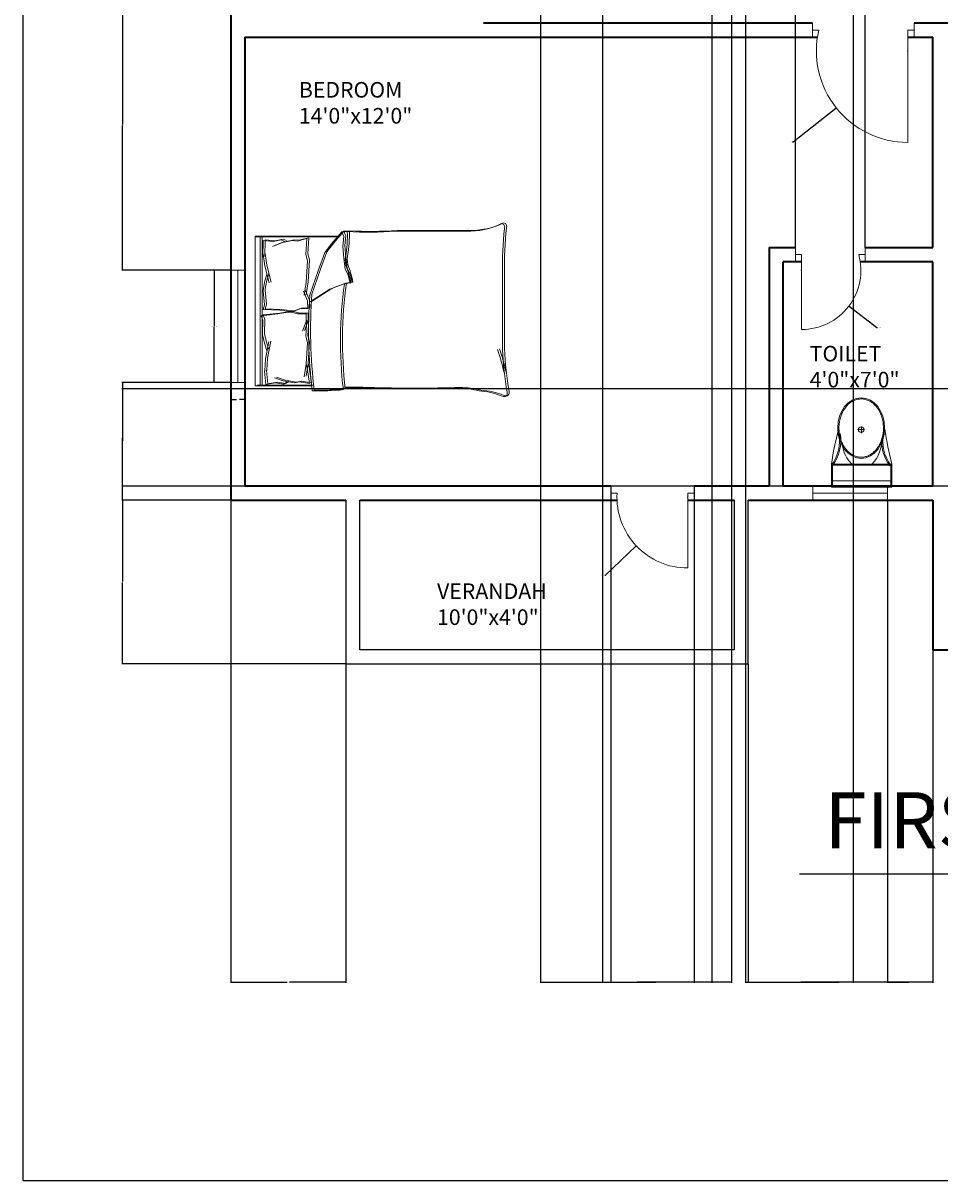
# Model space of a CAD drawing. Units: inches. Extents: x 1861 to 2564, y 1482 to 2317.
# Tile 1 of 11: x 1861 to 2155, y 1482 to 1853. Entities that reach past the tile are written whole.
import ezdxf

# ---------------------------------------------------------------- set-up
doc = ezdxf.new("R2010")
doc.units = ezdxf.units.IN
for name, color, linetype, lineweight in [('A-ANNO-DIMS', 2, 'Continuous', 18), ('A-ANNO-TEXT', 7, 'Continuous', 25), ('A-ANNO-TTLB', 7, 'Continuous', 25), ('A-AREA-IDEN', 7, 'Continuous', 18), ('A-DOOR', 3, 'Continuous', 18), ('A-FLOR-EDGE', 7, 'Continuous', 25), ('A-FLOR-FIXT', 8, 'Continuous', 18), ('A-FURN', 8, 'Continuous', 13), ('A-GLAZ', 4, 'Continuous', 18), ('A-WALL', 7, 'Continuous', 35)]:
    doc.layers.add(name, color=color, linetype=linetype, lineweight=lineweight)
doc.styles.get("Standard").update_dxf_attribs({"font": 'arial.ttf'})
doc.dimstyles.get("Standard").update_dxf_attribs({"dimtxt": 0.18, "dimasz": 0.18, "dimexe": 0.18, "dimexo": 0.0625, "dimgap": 0.09, "dimtad": 0, "dimtih": 1, "dimtoh": 1, "dimdec": 4, "dimzin": 0, "dimdsep": 46, "dimtxsty": 'Standard', "dimcen": 0.09, "dimadec": 0, "dimazin": 0, "dimtfac": 1, "dimtdec": 4, "dimtofl": 0, "dimtmove": 0, "dimatfit": 3, "dimfxl": 1, "dimtolj": 1, "dimtzin": 0, "dimarcsym": 0})

# ---------------------------------------------------------------- blocks, each defined once
blk = doc.blocks.new('A$C31115884')
for p, q in [((257.5, 466.4), (257.5, 523.2)), ((283.1, 497.7), (223.4, 497.7)), ((0, 200), (0, 0)), ((520, 200), (0, 200)), ((520, 0), (520, 200)), ((10, 190), (10, 10)), ((510, 190), (10, 190)), ((510, 10), (510, 190)), ((510, 54.5), (0, 54.5)), ((10, 10), (510, 10)), ((0, 0), (520, 0))]:
    blk.add_line(p, q)
blk.add_circle((255.6, 496.4), 23.6)
for centre, radius, start, end in [((2777.7, -204.6), 2807, 165.4549, 171.71327), ((3237, 905), 2807, 188.28673, 194.5451), ((-294.5, 403.3), 364.7, 324.20913, 9.34987), ((-294.5, 403.3), 374.7, 324.20913, 9.34987), ((139.5, 406.2), 293.5, 315.84364, 2.65635), ((805.8, 403.3), 374.7, 179.20365, 215.79087), ((805.8, 403.3), 364.7, 170.65013, 215.79087), ((383.6, 406.2), 293.5, 190.27735, 224.15636)]:
    blk.add_arc(centre, radius, start, end)
blk.add_ellipse((256.2, 509.9), major_axis=(0, -260.7), ratio=0.772727)
blk.add_open_spline([(256.2, 259.2), (263.1, 259.2), (270, 259.7), (287.8, 262.3), (298.7, 265.1), (319.9, 273.1), (330.2, 278.4), (350.1, 291.1), (359.7, 298.7), (377.7, 315.9), (386.2, 325.5), (401.7, 346.6), (408.8, 358.1), (421.3, 382.5), (426.8, 395.5), (435.9, 422.4), (439.5, 436.4), (444.8, 465.1), (446.5, 479.7), (447.9, 509.2), (447.6, 524), (445, 553.3), (442.7, 567.8), (436.3, 596), (432.1, 609.7), (421.9, 636), (416, 648.6), (402.5, 672.1), (395, 683), (378.6, 703), (369.8, 712.1), (351.1, 728), (341.3, 734.8), (320.9, 746.2), (310.4, 750.7), (288.9, 757.3), (278, 759.4), (256, 761), (245, 760.6), (223.1, 757.2), (212.3, 754.3), (191.1, 746.1), (180.8, 740.7), (160.9, 727.8), (151.4, 720.1), (133.5, 702.7), (125.1, 693), (109.6, 671.7), (102.6, 660.2), (90.2, 635.7), (84.9, 622.7), (76, 595.6), (72.4, 581.6), (67.2, 552.9), (65.6, 538.2), (64.4, 508.8), (64.8, 494), (67.5, 464.7), (69.9, 450.2), (76.6, 422), (80.8, 408.3), (91.1, 382.2), (97.2, 369.7), (110.8, 346.3), (118.4, 335.4), (134.8, 315.6), (143.7, 306.7), (162.4, 290.9), (172.3, 284.2), (192.8, 273), (203.3, 268.6), (224.8, 262.2), (235.8, 260.2), (249.9, 259.3), (253, 259.2), (256.2, 259.2)], degree=3, knots=[0, 0, 0, 0, 0.110105, 0.110105, 0.285049, 0.285049, 0.459994, 0.459994, 0.634938, 0.634938, 0.809882, 0.809882, 0.984827, 0.984827, 1.159771, 1.159771, 1.334715, 1.334715, 1.50966, 1.50966, 1.684604, 1.684604, 1.859549, 1.859549, 2.034493, 2.034493, 2.209437, 2.209437, 2.384382, 2.384382, 2.559326, 2.559326, 2.73427, 2.73427, 2.909215, 2.909215, 3.084159, 3.084159, 3.259103, 3.259103, 3.434048, 3.434048, 3.608992, 3.608992, 3.783936, 3.783936, 3.958881, 3.958881, 4.133825, 4.133825, 4.30877, 4.30877, 4.483714, 4.483714, 4.658658, 4.658658, 4.833603, 4.833603, 5.008547, 5.008547, 5.183491, 5.183491, 5.358436, 5.358436, 5.53338, 5.53338, 5.708324, 5.708324, 5.883269, 5.883269, 6.058213, 6.058213, 6.233158, 6.233158, 6.283185, 6.283185, 6.283185, 6.283185])
blk = doc.blocks.new('WIN-24IN')
for p, q in [((0, 24), (4.5, 24)), ((4.5, 24), (2.25, 24)), ((2.25, 24), (2.25, 0)), ((2.25, 0), (0, 0)), ((0, 0), (4.5, 0))]:
    blk.add_line(p, q)
blk = doc.blocks.new('WIN-36IN')
for p, q in [((0, 4.5), (0, 0)), ((36, 2.25), (36, 4.5)), ((36, 4.5), (36, 0)), ((0, 0), (0, 2.25)), ((0, 2.25), (36, 2.25))]:
    blk.add_line(p, q)
blk = doc.blocks.new('BED-DOUBLE')
for p, q in [((3.48, 63.34), (3.48, 81.45)), ((3.48, 63.34), (3.48, 81.45)), ((51.27, 81.45), (3.48, 81.45)), ((3.48, 79.91), (51.27, 79.91)), ((3.48, 79.91), (51.27, 79.91)), ((3.7, 62.7), (3.7, 80.81)), ((3.7, 62.7), (3.7, 80.81)), ((3.7, 79.27), (51.49, 79.27)), ((3.7, 79.27), (51.49, 79.27)), ((3.9, 78.11), (8.18, 78.44)), ((3.9, 78.11), (8.18, 78.44)), ((3.9, 78.13), (4.47, 74.95)), ((3.9, 78.13), (4.47, 74.95)), ((8.18, 78.44), (8.29, 78.42)), ((8.18, 78.44), (8.29, 78.42)), ((8.29, 78.42), (12.11, 78.13)), ((8.29, 78.42), (12.11, 78.13)), ((12.11, 78.13), (17.6, 77.12)), ((12.11, 78.13), (17.6, 77.12)), ((14.86, 77.7), (16.88, 78.42)), ((14.86, 77.7), (16.88, 78.42)), ((16.88, 78.42), (19.77, 79.14)), ((16.88, 78.42), (19.77, 79.14)), ((17.11, 77.78), (20, 78.5)), ((17.11, 77.78), (20, 78.5)), ((19.77, 79.14), (20.09, 79.14)), ((19.77, 79.14), (20.09, 79.14)), ((20, 78.5), (20.32, 78.5)), ((20, 78.5), (20.32, 78.5)), ((20.09, 79.14), (24.54, 79)), ((20.09, 79.14), (24.54, 79)), ((20.32, 78.5), (24.77, 78.36)), ((20.32, 78.5), (24.77, 78.36)), ((24.54, 79), (25.98, 79.58)), ((24.54, 79), (25.98, 79.58)), ((24.77, 78.36), (26.21, 78.94)), ((24.77, 78.36), (26.21, 78.94)), ((25.98, 79.58), (26.56, 74.23)), ((25.98, 79.58), (26.56, 74.23)), ((26.21, 78.94), (26.79, 73.59)), ((26.21, 78.94), (26.79, 73.59)), ((27.98, 78.95), (27.73, 73.58)), ((27.98, 78.95), (27.73, 73.58)), ((28.21, 78.31), (27.96, 72.94)), ((28.21, 78.31), (27.96, 72.94)), ((29.46, 78.47), (27.98, 78.95)), ((29.46, 78.47), (27.98, 78.95)), ((29.69, 77.83), (28.21, 78.31)), ((29.68, 77.83), (28.21, 78.31)), ((33.88, 78.89), (29.46, 78.47)), ((33.88, 78.89), (29.46, 78.47)), ((34.11, 78.25), (29.68, 77.83)), ((34.11, 78.25), (29.69, 77.83)), ((34.21, 78.91), (33.88, 78.89)), ((34.21, 78.91), (33.88, 78.89)), ((34.43, 78.27), (34.11, 78.25)), ((34.43, 78.27), (34.11, 78.25)), ((37.14, 78.37), (34.21, 78.91)), ((37.14, 78.37), (34.21, 78.91)), ((37.36, 77.73), (34.43, 78.27)), ((37.36, 77.73), (34.43, 78.27)), ((41.92, 78.38), (36.5, 77.02)), ((41.92, 78.38), (36.5, 77.02)), ((39.2, 77.77), (37.14, 78.37)), ((39.2, 77.77), (37.14, 78.37)), ((45.71, 78.9), (41.92, 78.38)), ((45.71, 78.9), (41.92, 78.38)), ((45.94, 78.26), (42.14, 77.74)), ((45.94, 78.26), (42.14, 77.74)), ((50.11, 78.89), (44.71, 78.99)), ((44.71, 78.99), (45.71, 78.9)), ((50.11, 78.89), (44.71, 78.99)), ((44.71, 78.99), (45.71, 78.9)), ((50.34, 78.25), (44.94, 78.35)), ((44.94, 78.35), (45.94, 78.26)), ((50.34, 78.25), (44.94, 78.35)), ((44.94, 78.35), (45.94, 78.26)), ((50.11, 78.89), (49.73, 75.68)), ((50.11, 78.89), (49.73, 75.68)), ((50.34, 78.25), (49.96, 75.04)), ((50.34, 78.25), (49.96, 75.04)), ((51.27, 81.45), (51.27, 54.84)), ((51.27, 81.45), (51.27, 54.84)), ((51.27, 81.45), (51.49, 81.45)), ((51.49, 81.45), (51.49, 80.81)), ((51.49, 80.81), (51.49, 54.2)), ((51.49, 80.81), (51.49, 54.2)), ((4.47, 74.95), (4.04, 72.35)), ((4.47, 74.95), (4.04, 72.35)), ((4.12, 77.49), (4.7, 74.31)), ((4.12, 77.49), (4.7, 74.31)), ((4.13, 77.47), (8.41, 77.8)), ((4.13, 77.47), (8.41, 77.8)), ((4.7, 74.31), (4.27, 71.71)), ((4.7, 74.31), (4.27, 71.71)), ((5.05, 72.49), (6.06, 75.24)), ((5.05, 72.49), (6.06, 75.24)), ((5.28, 71.85), (6.29, 74.6)), ((5.28, 71.85), (6.29, 74.6)), ((8.41, 77.8), (8.51, 77.78)), ((8.41, 77.8), (8.51, 77.78)), ((8.51, 77.78), (12.34, 77.49)), ((8.51, 77.78), (12.34, 77.49)), ((12.34, 77.49), (17.83, 76.48)), ((12.34, 77.49), (17.83, 76.48)), ((15.08, 77.06), (17.11, 77.78)), ((15.08, 77.06), (17.11, 77.78)), ((42.14, 77.74), (36.72, 76.38)), ((42.14, 77.74), (36.72, 76.38)), ((39.43, 77.13), (37.36, 77.73)), ((39.43, 77.13), (37.36, 77.73)), ((49.31, 73.19), (48.13, 75.87)), ((49.31, 73.19), (48.13, 75.87)), ((49.54, 72.55), (48.36, 75.23)), ((49.54, 72.55), (48.36, 75.23)), ((49.73, 75.68), (50.33, 73.11)), ((49.73, 75.68), (50.33, 73.11)), ((49.96, 75.04), (50.56, 72.47)), ((49.96, 75.04), (50.56, 72.47)), ((4.04, 72.35), (4.62, 71.33)), ((4.04, 72.35), (4.62, 71.33)), ((4.27, 71.71), (4.85, 70.69)), ((4.27, 71.71), (4.85, 70.69)), ((4.47, 68.88), (5.05, 72.49)), ((4.47, 68.88), (5.05, 72.49)), ((4.7, 68.24), (5.28, 71.85)), ((4.7, 68.24), (5.28, 71.85)), ((26.56, 74.23), (27.14, 71.04)), ((26.56, 74.23), (27.14, 71.04)), ((26.79, 73.59), (27.37, 70.41)), ((26.79, 73.59), (27.37, 70.41)), ((27.14, 71.04), (27.14, 69.74)), ((27.14, 71.04), (27.14, 69.74)), ((27.73, 73.58), (27.36, 70.37)), ((27.73, 73.58), (27.36, 70.37)), ((27.96, 72.94), (27.58, 69.73)), ((27.96, 72.94), (27.58, 69.73)), ((50.11, 69.62), (49.31, 73.19)), ((50.11, 69.62), (49.31, 73.19)), ((50.34, 68.98), (49.54, 72.55)), ((50.34, 68.98), (49.54, 72.55)), ((50.33, 73.11), (49.82, 72.06)), ((50.33, 73.11), (49.82, 72.06)), ((50.56, 72.47), (50.04, 71.42)), ((50.56, 72.47), (50.04, 71.42)), ((4.18, 64.1), (4.76, 67.29)), ((4.18, 64.1), (4.76, 67.29)), ((4.76, 67.29), (4.47, 68.88)), ((4.76, 67.29), (4.47, 68.88)), ((4.99, 66.65), (4.7, 68.24)), ((4.99, 66.65), (4.7, 68.24)), ((27.14, 69.74), (26.56, 67.86)), ((27.14, 69.74), (26.56, 67.86)), ((26.56, 67.86), (26.56, 65.18)), ((26.56, 67.86), (26.56, 65.18)), ((27.37, 69.1), (26.79, 67.22)), ((27.37, 69.1), (26.79, 67.22)), ((26.79, 67.22), (26.79, 64.54)), ((26.79, 67.22), (26.79, 64.54)), ((27.36, 70.37), (27.44, 69.07)), ((27.36, 70.37), (27.44, 69.07)), ((27.37, 70.41), (27.37, 69.1)), ((27.37, 70.41), (27.37, 69.1)), ((27.44, 69.07), (28.13, 67.23)), ((27.44, 69.07), (28.13, 67.23)), ((27.58, 69.73), (27.67, 68.43)), ((27.58, 69.73), (27.67, 68.43)), ((27.67, 68.43), (28.36, 66.59)), ((27.67, 68.43), (28.36, 66.59)), ((28.13, 67.23), (28.3, 64.55)), ((28.13, 67.23), (28.3, 64.55)), ((49.92, 68.01), (50.11, 69.62)), ((49.92, 68.01), (50.11, 69.62)), ((50.7, 64.87), (49.92, 68.01)), ((50.7, 64.87), (49.92, 68.01)), ((50.15, 67.37), (50.34, 68.98)), ((50.15, 67.37), (50.34, 68.98)), ((50.93, 64.23), (50.15, 67.37)), ((50.93, 64.23), (50.15, 67.37)), ((9.28, 64.83), (4.18, 64.1)), ((9.28, 64.83), (4.18, 64.1)), ((4.41, 63.46), (4.99, 66.65)), ((4.41, 63.46), (4.99, 66.65)), ((9.51, 64.19), (4.41, 63.46)), ((9.51, 64.19), (4.41, 63.46)), ((6.38, 65.82), (10.41, 65.15)), ((6.38, 65.82), (10.41, 65.15)), ((6.61, 65.18), (10.64, 64.51)), ((6.61, 65.18), (10.64, 64.51)), ((10.41, 65.15), (9.28, 64.83)), ((10.41, 65.15), (9.28, 64.83)), ((10.64, 64.51), (9.51, 64.19)), ((10.64, 64.51), (9.51, 64.19)), ((10.41, 65.15), (17.42, 64.72)), ((10.41, 65.15), (17.42, 64.72)), ((10.64, 64.51), (17.65, 64.08)), ((10.64, 64.51), (17.65, 64.08)), ((17.42, 64.72), (19.38, 65.28)), ((17.42, 64.72), (19.38, 65.28)), ((17.65, 64.08), (19.61, 64.64)), ((17.65, 64.08), (19.61, 64.64)), ((19.38, 65.28), (24.52, 64.87)), ((19.38, 65.28), (24.52, 64.87)), ((19.61, 64.64), (24.75, 64.23)), ((19.61, 64.64), (24.74, 64.23)), ((24.1, 65.18), (20.96, 66.27)), ((24.1, 65.18), (20.96, 66.27)), ((24.33, 64.54), (21.19, 65.63)), ((24.33, 64.54), (21.19, 65.63)), ((26.56, 65.18), (24.1, 65.18)), ((26.56, 65.18), (24.1, 65.18)), ((26.79, 64.54), (24.33, 64.54)), ((26.79, 64.54), (24.33, 64.54)), ((28.3, 64.55), (30.75, 64.71)), ((28.3, 64.55), (30.75, 64.71)), ((28.36, 66.59), (28.53, 63.91)), ((28.36, 66.59), (28.53, 63.91)), ((28.53, 63.91), (30.98, 64.07)), ((28.53, 63.91), (30.98, 64.07)), ((30.26, 64.06), (34.45, 57.57)), ((30.26, 64.06), (34.45, 57.57)), ((30.49, 63.42), (34.68, 56.93)), ((30.49, 63.42), (34.68, 56.93)), ((30.75, 64.71), (33.82, 65.99)), ((30.75, 64.71), (33.82, 65.99)), ((30.98, 64.07), (34.05, 65.35)), ((30.98, 64.07), (34.05, 65.35)), ((40.65, 61.13), (32.31, 64.06)), ((40.64, 61.13), (32.31, 64.06)), ((40.87, 60.49), (32.54, 63.42)), ((40.87, 60.49), (32.54, 63.42)), ((32.56, 65.82), (36.6, 65.15)), ((32.57, 65.82), (36.6, 65.15)), ((32.79, 65.18), (36.83, 64.51)), ((32.79, 65.18), (36.83, 64.51)), ((36.6, 65.15), (43.61, 64.72)), ((36.6, 65.15), (43.61, 64.72)), ((36.83, 64.51), (43.84, 64.08)), ((36.83, 64.51), (43.84, 64.08)), ((43.61, 64.72), (45.57, 65.28)), ((43.61, 64.72), (45.57, 65.28)), ((43.84, 64.08), (45.8, 64.64)), ((43.84, 64.08), (45.8, 64.64)), ((45.57, 65.28), (50.7, 64.87)), ((45.57, 65.28), (50.7, 64.87)), ((45.8, 64.64), (50.93, 64.23)), ((45.8, 64.64), (50.93, 64.23)), ((46.22, 59.12), (40.64, 61.13)), ((46.22, 59.12), (40.65, 61.13)), ((46.45, 58.48), (40.87, 60.49)), ((46.45, 58.48), (40.87, 60.49)), ((34.45, 57.57), (36.15, 53.08)), ((34.45, 57.57), (36.15, 53.08)), ((34.68, 56.93), (36.38, 52.44)), ((34.68, 56.93), (36.38, 52.44)), ((49.16, 56.95), (46.22, 59.12)), ((49.16, 56.95), (46.22, 59.12)), ((49.39, 56.31), (46.45, 58.48)), ((49.39, 56.31), (46.45, 58.48)), ((52.87, 53.7), (49.16, 56.95)), ((52.87, 53.7), (49.16, 56.95)), ((53.1, 53.06), (49.39, 56.31)), ((53.1, 53.06), (49.39, 56.31)), ((36.15, 53.08), (36.46, 51.07)), ((36.15, 53.08), (36.46, 51.07)), ((36.38, 52.44), (36.69, 50.43)), ((36.38, 52.44), (36.69, 50.43)), ((38.94, 51.69), (40.95, 52.62)), ((38.94, 51.69), (40.95, 52.62)), ((40.95, 52.62), (44.36, 53.08)), ((40.95, 52.62), (44.36, 53.08)), ((41.18, 51.98), (44.59, 52.44)), ((41.18, 51.98), (44.59, 52.44)), ((44.36, 53.08), (48.23, 53.39)), ((44.36, 53.08), (48.23, 53.39)), ((44.59, 52.44), (48.46, 52.75)), ((44.59, 52.44), (48.46, 52.75)), ((48.23, 53.39), (51.33, 53.08)), ((48.23, 53.39), (51.33, 53.08)), ((48.46, 52.75), (51.56, 52.44)), ((48.46, 52.75), (51.56, 52.44)), ((51.33, 53.08), (52.87, 53.7)), ((51.33, 53.08), (52.87, 53.7)), ((51.56, 52.44), (53.1, 53.06)), ((51.56, 52.44), (53.1, 53.06)), ((52.95, 51.95), (52.87, 53.7, 3.87)), ((52.95, 51.95), (52.87, 53.7, 3.87)), ((53.18, 51.32), (53.1, 53.06, 3.87)), ((53.18, 51.32), (53.1, 53.06, 3.87)), ((36.46, 51.07), (38.94, 51.69)), ((36.46, 51.07), (38.94, 51.69)), ((36.69, 50.43), (39.17, 51.05)), ((36.69, 50.43), (39.17, 51.05)), ((39.17, 51.05), (41.18, 51.98)), ((39.17, 51.05), (41.18, 51.98)), ((15.06, 2.2), (39.68, 2.2)), ((15.06, 2.2), (39.68, 2.2)), ((15.29, 1.56), (39.91, 1.56)), ((15.29, 1.56), (39.91, 1.56))]:
    blk.add_line(p, q)
for centre, radius, start, end in [((85.16, 61.35), 83.31, 178.7218, 185.604), ((85.16, 61.35), 83.31, 178.7218, 185.604), ((21.36, -100.61), 164.97, 86.0865, 96.7821), ((21.36, -100.61), 164.97, 86.0865, 96.7821), ((21.59, -101.25), 164.97, 86.0865, 96.7821), ((21.59, -101.25), 164.97, 86.0865, 96.7821), ((85.39, 60.71), 83.31, 178.7218, 185.604), ((85.39, 60.71), 83.31, 178.7218, 185.604), ((17.76, -74.87), 129.02, 81.7845, 96.9006), ((17.76, -74.87), 129.02, 81.7845, 96.9006), ((17.99, -75.51), 129.02, 81.7845, 96.9006), ((17.98, -75.51), 129.02, 81.7845, 96.9006), ((-167.31, 50.27), 170.11, 358.4762, 1.0082), ((-167.31, 50.27), 170.11, 358.4762, 1.0082), ((-167.08, 49.63), 170.11, 358.4762, 1.0082), ((-167.08, 49.63), 170.11, 358.4762, 1.0082), ((31.15, 79.96), 29.65, 280.6617, 289.8806), ((31.15, 79.96), 29.65, 280.6617, 289.8806), ((43.74, 46.38), 6.22, 78.6608, 113.7384), ((43.74, 46.38), 6.22, 78.6608, 113.7384), ((51.33, 88.1), 36.18, 259.8763, 272.5657), ((51.33, 88.1), 36.18, 259.8763, 272.5657), ((36.64, 51.01), 0.185, 160.2464, 271.1377), ((36.64, 51.01), 0.185, 160.2464, 271.1377), ((36.87, 50.37), 0.185, 160.2464, 271.1377), ((36.87, 50.37), 0.185, 160.2464, 271.1377), ((31.38, 79.32), 29.65, 280.6617, 289.8806), ((31.38, 79.32), 29.65, 280.6617, 289.8806), ((43.97, 45.74), 6.22, 78.6608, 113.7384), ((43.97, 45.74), 6.22, 78.6608, 113.7384), ((51.56, 87.46), 36.18, 259.8763, 272.5657), ((51.56, 87.46), 36.18, 259.8763, 272.5657), ((182.27, 45.13), 129.5, 176.9791, 183.8365), ((182.27, 45.13), 129.5, 176.9791, 183.8365), ((182.5, 44.49), 129.5, 176.9791, 183.8365), ((182.49, 44.49), 129.5, 176.9791, 183.8365), ((484.82, 30.83), 482.31, 178.2277, 181.7185), ((484.82, 30.83), 482.31, 178.2277, 181.7185), ((485.05, 30.19), 482.31, 178.2277, 181.7185), ((485.05, 30.19), 482.31, 178.2277, 181.7185), ((-4508.74, 13.62), 4561.86, 0.00217, 0.28689), ((-4508.74, 13.62), 4561.86, 0.00217, 0.28689), ((-4508.51, 12.98), 4561.86, 0.00217, 0.28689), ((-4508.51, 12.98), 4561.86, 0.00217, 0.28689), ((-26.9, 16.93), 29.63, 346.0648, 358.9113), ((-26.9, 16.93), 29.63, 346.0648, 358.9113), ((-26.67, 16.29), 29.63, 346.0648, 358.9113), ((-26.67, 16.29), 29.63, 346.0648, 358.9113), ((76.16, 12.78), 23.07, 177.4714, 206.4681), ((76.16, 12.78), 23.07, 177.4714, 206.4681), ((76.39, 12.14), 23.07, 177.4714, 206.4681), ((76.39, 12.14), 23.07, 177.4714, 206.4681), ((-21.66, 11.17), 23.56, 337.9751, 356.652), ((-21.66, 11.17), 23.56, 337.9751, 356.652), ((-21.43, 10.53), 23.56, 337.9751, 356.652), ((-21.43, 10.53), 23.56, 337.9751, 356.652), ((-17.22, 105.16), 106.46, 283.3832, 287.7053), ((-17.22, 105.16), 106.46, 283.3832, 287.7053), ((1.09, 1.73), 1.09, 146.1736, 293.4781), ((1.09, 1.73), 1.09, 146.1736, 293.4781), ((1.32, 1.09), 1.09, 146.1736, 293.4781), ((1.32, 1.09), 1.09, 146.1736, 293.4781), ((21.43, -119.39), 121.76, 92.9958, 99.4091), ((21.43, -119.39), 121.76, 92.9958, 99.4091), ((21.66, -120.03), 121.76, 92.9958, 99.4091), ((21.66, -120.03), 121.76, 92.9958, 99.4091), ((-16.99, 104.52), 106.46, 283.3832, 287.7053), ((-16.99, 104.52), 106.46, 283.3832, 287.7053), ((41.15, -130.83), 133.04, 84.4998, 90.6351), ((41.15, -130.83), 133.04, 84.4998, 90.6351), ((41.38, -131.47), 133.04, 84.4998, 90.6351), ((41.38, -131.47), 133.04, 84.4998, 90.6351), ((54.41, 2.58), 1.1, 242.6588, 356.02), ((54.41, 2.58), 1.1, 242.6588, 356.02), ((54.64, 1.94), 1.1, 242.6588, 356.02), ((54.64, 1.94), 1.1, 242.6588, 356.02)]:
    blk.add_arc(centre, radius, start, end)
blk = doc.blocks.new('*D18')
at = {"layer": 'A-ANNO-DIMS', "color": 0, "lineweight": -2, "transparency": 16777216}
for p, q in [((1927.68, 1774.13), (1922.16, 1774.13)), ((1922.34, 1773.95), (1922.34, 1756.32)), ((1922.34, 1738.31), (1922.34, 1755.95)), ((1927.68, 1738.13), (1922.16, 1738.13))]:
    blk.add_line(p, q, dxfattribs=at)
at = {"layer": 'A-ANNO-DIMS', "color": 0, "transparency": 16777216}
for points in [[(1922.31, 1773.95), (1922.37, 1773.95), (1922.34, 1774.13)], [(1922.31, 1738.31), (1922.37, 1738.31), (1922.34, 1738.13)]]:
    blk.add_solid(points, dxfattribs=at)
at = {"layer": 'Defpoints', "color": 0, "transparency": 16777216}
for p in [(1927.74, 1774.13), (1922.34, 1738.13), (1927.74, 1738.13)]:
    blk.add_point(p, dxfattribs=at)
at = {"layer": 'A-ANNO-DIMS', "color": 0, "transparency": 16777216, "insert": (1922.34, 1756.13), "char_height": 0.18, "attachment_point": 5}
blk.add_mtext('\\A1;WINDOW 36 TYP.', dxfattribs=at)
blk = doc.blocks.new('*D19')
at = {"layer": 'A-ANNO-DIMS', "color": 0, "lineweight": -2, "transparency": 16777216}
for p, q in [((1927.74, 1738.07), (1927.74, 1732.55)), ((1932.24, 1738.07), (1932.24, 1732.55)), ((1927.92, 1732.73), (1929.53, 1732.73)), ((1932.06, 1732.73), (1930.45, 1732.73))]:
    blk.add_line(p, q, dxfattribs=at)
at = {"layer": 'A-ANNO-DIMS', "color": 0, "transparency": 16777216}
for points in [[(1927.92, 1732.76), (1927.92, 1732.7), (1927.74, 1732.73)], [(1932.06, 1732.76), (1932.06, 1732.7), (1932.24, 1732.73)]]:
    blk.add_solid(points, dxfattribs=at)
at = {"layer": 'Defpoints', "color": 0, "transparency": 16777216}
for p in [(1927.74, 1738.13), (1932.24, 1738.13), (1932.24, 1732.73)]:
    blk.add_point(p, dxfattribs=at)
at = {"layer": 'A-ANNO-DIMS', "color": 0, "transparency": 16777216, "insert": (1929.99, 1732.73), "char_height": 0.18, "attachment_point": 5}
blk.add_mtext('\\A1;5 TYP.', dxfattribs=at)
blk = doc.blocks.new('*D35')
at = {"layer": 'A-ANNO-DIMS', "color": 0, "lineweight": -2, "transparency": 16777216}
for p, q in [((2026.99, 2250.82), (2026.99, 1545.6)), ((2088.24, 2250.82), (2088.24, 1545.6)), ((2027.17, 1545.78), (2057.22, 1545.78)), ((2088.06, 1545.78), (2058.01, 1545.78))]:
    blk.add_line(p, q, dxfattribs=at)
at = {"layer": 'A-ANNO-DIMS', "color": 0, "transparency": 16777216}
for points in [[(2027.17, 1545.81), (2027.17, 1545.75), (2026.99, 1545.78)], [(2088.06, 1545.81), (2088.06, 1545.75), (2088.24, 1545.78)]]:
    blk.add_solid(points, dxfattribs=at)
at = {"layer": 'Defpoints', "color": 0, "transparency": 16777216}
for p in [(2026.99, 2250.89), (2088.24, 2250.89), (2088.24, 1545.78)]:
    blk.add_point(p, dxfattribs=at)
at = {"layer": 'A-ANNO-DIMS', "color": 0, "transparency": 16777216, "insert": (2057.61, 1545.78), "char_height": 0.18, "attachment_point": 5}
blk.add_mtext('\\A1;61.25', dxfattribs=at)
blk = doc.blocks.new('*D36')
at = {"layer": 'A-ANNO-DIMS', "color": 0, "lineweight": -2, "transparency": 16777216}
for p, q in [((2092.74, 2250.82), (2092.74, 1545.6)), ((2127.18, 2250.82), (2127.18, 1545.6)), ((2092.92, 1545.78), (2109.5, 1545.78)), ((2127, 1545.78), (2110.43, 1545.78))]:
    blk.add_line(p, q, dxfattribs=at)
at = {"layer": 'A-ANNO-DIMS', "color": 0, "transparency": 16777216}
for points in [[(2092.92, 1545.81), (2092.92, 1545.75), (2092.74, 1545.78)], [(2127, 1545.81), (2127, 1545.75), (2127.18, 1545.78)]]:
    blk.add_solid(points, dxfattribs=at)
at = {"layer": 'Defpoints', "color": 0, "transparency": 16777216}
for p in [(2092.74, 2250.89), (2127.18, 2250.89), (2127.18, 1545.78)]:
    blk.add_point(p, dxfattribs=at)
at = {"layer": 'A-ANNO-DIMS', "color": 0, "transparency": 16777216, "insert": (2109.96, 1545.78), "char_height": 0.18, "attachment_point": 5}
blk.add_mtext('\\A1;34.445', dxfattribs=at)
blk = doc.blocks.new('*D43')
at = {"layer": 'A-ANNO-DIMS', "color": 0, "lineweight": -2, "transparency": 16777216}
for p, q in [((1927.68, 1867.33), (1892.76, 1867.33)), ((1892.94, 1867.15), (1892.94, 1820.91)), ((1892.94, 1774.31), (1892.94, 1820.55)), ((1927.68, 1774.13), (1892.76, 1774.13))]:
    blk.add_line(p, q, dxfattribs=at)
at = {"layer": 'A-ANNO-DIMS', "color": 0, "transparency": 16777216}
for points in [[(1892.91, 1867.15), (1892.97, 1867.15), (1892.94, 1867.33)], [(1892.91, 1774.31), (1892.97, 1774.31), (1892.94, 1774.13)]]:
    blk.add_solid(points, dxfattribs=at)
at = {"layer": 'Defpoints', "color": 0, "transparency": 16777216}
for p in [(1927.74, 1867.33), (1892.94, 1774.13), (1927.74, 1774.13)]:
    blk.add_point(p, dxfattribs=at)
at = {"layer": 'A-ANNO-DIMS', "color": 0, "transparency": 16777216, "insert": (1892.94, 1820.73), "char_height": 0.18, "attachment_point": 5}
blk.add_mtext('\\A1;93.19', dxfattribs=at)
blk = doc.blocks.new('*D44')
at = {"layer": 'A-ANNO-DIMS', "color": 0, "lineweight": -2, "transparency": 16777216}
for p, q in [((1927.68, 1738.13), (1892.76, 1738.13)), ((1892.94, 1737.95), (1892.94, 1719.44)), ((1892.94, 1700.57), (1892.94, 1719.08)), ((1927.68, 1700.39), (1892.76, 1700.39))]:
    blk.add_line(p, q, dxfattribs=at)
at = {"layer": 'A-ANNO-DIMS', "color": 0, "transparency": 16777216}
for points in [[(1892.91, 1737.95), (1892.97, 1737.95), (1892.94, 1738.13)], [(1892.91, 1700.57), (1892.97, 1700.57), (1892.94, 1700.39)]]:
    blk.add_solid(points, dxfattribs=at)
at = {"layer": 'Defpoints', "color": 0, "transparency": 16777216}
for p in [(1927.74, 1738.13), (1892.94, 1700.39), (1927.74, 1700.39)]:
    blk.add_point(p, dxfattribs=at)
at = {"layer": 'A-ANNO-DIMS', "color": 0, "transparency": 16777216, "insert": (1892.94, 1719.26), "char_height": 0.18, "attachment_point": 5}
blk.add_mtext('\\A1;37.75', dxfattribs=at)
blk = doc.blocks.new('*D46')
at = {"layer": 'A-ANNO-DIMS', "color": 0, "lineweight": -2, "transparency": 16777216}
for p, q in [((1927.74, 1700.32), (1927.74, 1545.6)), ((1964.57, 1647.82), (1964.57, 1545.6)), ((1927.92, 1545.78), (1945.76, 1545.78)), ((1964.39, 1545.78), (1946.55, 1545.78))]:
    blk.add_line(p, q, dxfattribs=at)
at = {"layer": 'A-ANNO-DIMS', "color": 0, "transparency": 16777216}
for points in [[(1927.92, 1545.81), (1927.92, 1545.75), (1927.74, 1545.78)], [(1964.39, 1545.81), (1964.39, 1545.75), (1964.57, 1545.78)]]:
    blk.add_solid(points, dxfattribs=at)
at = {"layer": 'Defpoints', "color": 0, "transparency": 16777216}
for p in [(1927.74, 1700.39), (1964.57, 1647.89), (1964.57, 1545.78)]:
    blk.add_point(p, dxfattribs=at)
at = {"layer": 'A-ANNO-DIMS', "color": 0, "transparency": 16777216, "insert": (1946.16, 1545.78), "char_height": 0.18, "attachment_point": 5}
blk.add_mtext('\\A1;36.83', dxfattribs=at)
blk = doc.blocks.new('*D47')
at = {"layer": 'A-ANNO-DIMS', "color": 0, "lineweight": -2, "transparency": 16777216}
for p, q in [((2152.74, 1652.32), (2152.74, 1545.6)), ((2093.57, 1647.82), (2093.57, 1545.6)), ((2093.75, 1545.78), (2122.76, 1545.78)), ((2152.56, 1545.78), (2123.55, 1545.78))]:
    blk.add_line(p, q, dxfattribs=at)
at = {"layer": 'A-ANNO-DIMS', "color": 0, "transparency": 16777216}
for points in [[(2093.75, 1545.81), (2093.75, 1545.75), (2093.57, 1545.78)], [(2152.56, 1545.81), (2152.56, 1545.75), (2152.74, 1545.78)]]:
    blk.add_solid(points, dxfattribs=at)
at = {"layer": 'Defpoints', "color": 0, "transparency": 16777216}
for p in [(2152.74, 1652.39), (2093.57, 1647.89), (2152.74, 1545.78)]:
    blk.add_point(p, dxfattribs=at)
at = {"layer": 'A-ANNO-DIMS', "color": 0, "transparency": 16777216, "insert": (2123.16, 1545.78), "char_height": 0.18, "attachment_point": 5}
blk.add_mtext('\\A1;59.17', dxfattribs=at)
blk = doc.blocks.new('*D50')
at = {"layer": 'A-ANNO-DIMS', "color": 0, "lineweight": -2, "transparency": 16777216}
for p, q in [((1927.68, 1700.39), (1892.76, 1700.39)), ((1892.94, 1700.21), (1892.94, 1674.32)), ((1892.94, 1648.07), (1892.94, 1673.95)), ((1964.51, 1647.89), (1892.76, 1647.89))]:
    blk.add_line(p, q, dxfattribs=at)
at = {"layer": 'A-ANNO-DIMS', "color": 0, "transparency": 16777216}
for points in [[(1892.91, 1700.21), (1892.97, 1700.21), (1892.94, 1700.39)], [(1892.91, 1648.07), (1892.97, 1648.07), (1892.94, 1647.89)]]:
    blk.add_solid(points, dxfattribs=at)
at = {"layer": 'Defpoints', "color": 0, "transparency": 16777216}
for p in [(1892.94, 1700.39), (1927.74, 1700.39), (1964.57, 1647.89)]:
    blk.add_point(p, dxfattribs=at)
at = {"layer": 'A-ANNO-DIMS', "color": 0, "transparency": 16777216, "insert": (1892.94, 1674.14), "char_height": 0.18, "attachment_point": 5}
blk.add_mtext('\\A1;52.5', dxfattribs=at)
blk = doc.blocks.new('*D51')
at = {"layer": 'A-ANNO-DIMS', "color": 0, "lineweight": -2, "transparency": 16777216}
for p, q in [((2046.87, 2106.82), (2046.87, 1545.6)), ((2081.9, 2106.82), (2081.9, 1545.6)), ((2047.05, 1545.78), (2063.92, 1545.78)), ((2081.72, 1545.78), (2064.85, 1545.78))]:
    blk.add_line(p, q, dxfattribs=at)
at = {"layer": 'A-ANNO-DIMS', "color": 0, "transparency": 16777216}
for points in [[(2047.05, 1545.81), (2047.05, 1545.75), (2046.87, 1545.78)], [(2081.72, 1545.81), (2081.72, 1545.75), (2081.9, 1545.78)]]:
    blk.add_solid(points, dxfattribs=at)
at = {"layer": 'Defpoints', "color": 0, "transparency": 16777216}
for p in [(2046.87, 2106.89), (2081.9, 2106.89), (2081.9, 1545.78)]:
    blk.add_point(p, dxfattribs=at)
at = {"layer": 'A-ANNO-DIMS', "color": 0, "transparency": 16777216, "insert": (2064.39, 1545.78), "char_height": 0.18, "attachment_point": 5}
blk.add_mtext('\\A1;35.035', dxfattribs=at)
blk = doc.blocks.new('*D57')
at = {"layer": 'A-ANNO-DIMS', "color": 0, "lineweight": -2, "transparency": 16777216}
for p, q in [((2049.51, 1704.82), (2049.51, 1545.6)), ((2076.21, 1704.82), (2076.21, 1545.6)), ((2049.69, 1545.78), (2062.53, 1545.78)), ((2076.03, 1545.78), (2063.18, 1545.78))]:
    blk.add_line(p, q, dxfattribs=at)
at = {"layer": 'A-ANNO-DIMS', "color": 0, "transparency": 16777216}
for points in [[(2049.69, 1545.81), (2049.69, 1545.75), (2049.51, 1545.78)], [(2076.03, 1545.81), (2076.03, 1545.75), (2076.21, 1545.78)]]:
    blk.add_solid(points, dxfattribs=at)
at = {"layer": 'Defpoints', "color": 0, "transparency": 16777216}
for p in [(2049.51, 1704.89), (2076.21, 1704.89), (2076.21, 1545.78)]:
    blk.add_point(p, dxfattribs=at)
at = {"layer": 'A-ANNO-DIMS', "color": 0, "transparency": 16777216, "insert": (2062.86, 1545.78), "char_height": 0.18, "attachment_point": 5}
blk.add_mtext('\\A1;26.7', dxfattribs=at)
blk = doc.blocks.new('*D62')
at = {"layer": 'A-ANNO-DIMS', "color": 0, "lineweight": -2, "transparency": 16777216}
for p, q in [((2108.68, 1781.45), (2108.68, 2290.37)), ((2108.86, 2290.19), (2119.46, 2290.19)), ((2130.84, 2290.19), (2120.25, 2290.19)), ((2131.02, 1781.45), (2131.02, 2290.37))]:
    blk.add_line(p, q, dxfattribs=at)
at = {"layer": 'A-ANNO-DIMS', "color": 0, "transparency": 16777216}
for points in [[(2108.86, 2290.22), (2108.86, 2290.16), (2108.68, 2290.19)], [(2130.84, 2290.22), (2130.84, 2290.16), (2131.02, 2290.19)]]:
    blk.add_solid(points, dxfattribs=at)
at = {"layer": 'Defpoints', "color": 0, "transparency": 16777216}
for p in [(2131.02, 2290.19), (2108.68, 1781.39), (2131.02, 1781.39)]:
    blk.add_point(p, dxfattribs=at)
at = {"layer": 'A-ANNO-DIMS', "color": 0, "transparency": 16777216, "insert": (2119.85, 2290.19), "char_height": 0.18, "attachment_point": 5}
blk.add_mtext('\\A1;22.34', dxfattribs=at)
blk = doc.blocks.new('*D67')
at = {"layer": 'A-ANNO-DIMS', "color": 0, "lineweight": -2, "transparency": 16777216}
for p, q in [((2497.68, 1736.13), (1892.76, 1736.13)), ((1892.94, 1735.95), (1892.94, 1720.69)), ((1892.94, 1705.07), (1892.94, 1720.32)), ((2497.68, 1704.89), (1892.76, 1704.89))]:
    blk.add_line(p, q, dxfattribs=at)
at = {"layer": 'A-ANNO-DIMS', "color": 0, "transparency": 16777216}
for points in [[(1892.91, 1735.95), (1892.97, 1735.95), (1892.94, 1736.13)], [(1892.91, 1705.07), (1892.97, 1705.07), (1892.94, 1704.89)]]:
    blk.add_solid(points, dxfattribs=at)
at = {"layer": 'Defpoints', "color": 0, "transparency": 16777216}
for p in [(1892.94, 1736.13), (2497.74, 1736.13), (2497.74, 1704.89)]:
    blk.add_point(p, dxfattribs=at)
at = {"layer": 'A-ANNO-DIMS', "color": 0, "transparency": 16777216, "insert": (1892.94, 1720.51), "char_height": 0.18, "attachment_point": 5}
blk.add_mtext('\\A1;31.24', dxfattribs=at)
blk = doc.blocks.new('*D72')
at = {"layer": 'A-ANNO-DIMS', "color": 0, "lineweight": -2, "transparency": 16777216}
for p, q in [((2138.24, 1700.32), (2138.24, 1545.6)), ((2152.74, 1700.32), (2152.74, 1545.6)), ((2138.42, 1545.78), (2145.04, 1545.78)), ((2152.56, 1545.78), (2145.95, 1545.78))]:
    blk.add_line(p, q, dxfattribs=at)
at = {"layer": 'A-ANNO-DIMS', "color": 0, "transparency": 16777216}
for points in [[(2138.42, 1545.81), (2138.42, 1545.75), (2138.24, 1545.78)], [(2152.56, 1545.81), (2152.56, 1545.75), (2152.74, 1545.78)]]:
    blk.add_solid(points, dxfattribs=at)
at = {"layer": 'Defpoints', "color": 0, "transparency": 16777216}
for p in [(2138.24, 1700.39), (2152.74, 1700.39), (2152.74, 1545.78)]:
    blk.add_point(p, dxfattribs=at)
at = {"layer": 'A-ANNO-DIMS', "color": 0, "transparency": 16777216, "insert": (2145.49, 1545.78), "char_height": 0.18, "attachment_point": 5}
blk.add_mtext('\\A1;14.495', dxfattribs=at)
blk = doc.blocks.new('*D79')
at = {"layer": 'A-ANNO-DIMS', "color": 0, "lineweight": -2, "transparency": 16777216}
for p, q in [((2144.65, 1844.47), (2144.83, 1844.47)), ((2144.74, 1844.38), (2144.74, 1844.56)), ((2107.98, 1815.3), (2121.62, 1826.12)), ((2107.8, 1815.3), (2107.98, 1815.3))]:
    blk.add_line(p, q, dxfattribs=at)
at = {"layer": 'A-ANNO-DIMS', "color": 0, "transparency": 16777216}
blk.add_solid([(2121.61, 1826.15), (2121.64, 1826.1), (2121.76, 1826.24)], dxfattribs=at)
at = {"layer": 'Defpoints', "color": 0, "transparency": 16777216}
for p in [(2144.74, 1844.47), (2121.76, 1826.24)]:
    blk.add_point(p, dxfattribs=at)
at = {"layer": 'A-ANNO-DIMS', "color": 0, "transparency": 16777216, "insert": (2107.32, 1815.3), "char_height": 0.18, "attachment_point": 5}
blk.add_mtext('\\A1;R29.33', dxfattribs=at)
blk = doc.blocks.new('*D84')
at = {"layer": 'A-ANNO-DIMS', "color": 0, "lineweight": -2, "transparency": 16777216}
for p, q in [((2074.12, 1701.37), (2074.3, 1701.37)), ((2074.21, 1701.28), (2074.21, 1701.46)), ((2047.78, 1676.38), (2057.56, 1685.62)), ((2047.6, 1676.38), (2047.78, 1676.38))]:
    blk.add_line(p, q, dxfattribs=at)
at = {"layer": 'A-ANNO-DIMS', "color": 0, "transparency": 16777216}
blk.add_solid([(2057.54, 1685.65), (2057.58, 1685.6), (2057.69, 1685.75)], dxfattribs=at)
at = {"layer": 'Defpoints', "color": 0, "transparency": 16777216}
for p in [(2074.21, 1701.37), (2057.69, 1685.75)]:
    blk.add_point(p, dxfattribs=at)
at = {"layer": 'A-ANNO-DIMS', "color": 0, "transparency": 16777216, "insert": (2047.05, 1676.38), "char_height": 0.18, "attachment_point": 5}
blk.add_mtext('\\A1;R22.733', dxfattribs=at)
blk = doc.blocks.new('*D88')
at = {"layer": 'A-ANNO-DIMS', "color": 0, "lineweight": -2, "transparency": 16777216}
for p, q in [((2110.59, 1774.14), (2110.77, 1774.14)), ((2110.68, 1774.05), (2110.68, 1774.23)), ((2134.84, 1755.68), (2125.93, 1762.49)), ((2135.02, 1755.68), (2134.84, 1755.68))]:
    blk.add_line(p, q, dxfattribs=at)
at = {"layer": 'A-ANNO-DIMS', "color": 0, "transparency": 16777216}
blk.add_solid([(2125.94, 1762.52), (2125.91, 1762.47), (2125.78, 1762.6)], dxfattribs=at)
at = {"layer": 'Defpoints', "color": 0, "transparency": 16777216}
for p in [(2110.68, 1774.14), (2125.78, 1762.6)]:
    blk.add_point(p, dxfattribs=at)
at = {"layer": 'A-ANNO-DIMS', "color": 0, "transparency": 16777216, "insert": (2135.57, 1755.68), "char_height": 0.18, "attachment_point": 5}
blk.add_mtext('\\A1;R19.006', dxfattribs=at)

msp = doc.modelspace()

# ---------------------------------------------------------------- linework, layer by layer
at = {"layer": 'A-ANNO-TTLB'}
msp.add_line((2110.0229, 1580.5777), (2362.3195, 1580.5777), dxfattribs=at)
msp.add_lwpolyline([(1861.1332, 2316.6589), (2563.8077, 2316.6589), (2563.8077, 1482.0728), (1861.1332, 1482.0728)], close=True, dxfattribs=at)
at = {"layer": 'A-DOOR'}
for p, q in [((2114.1781, 1853.3854), (2114.1781, 1848.8854)), ((2146.7425, 1848.8854), (2146.7425, 1853.3854)), ((2146.7425, 1853.3854), (2146.7425, 1851.1354)), ((2114.1781, 1848.8854), (2114.1781, 1851.1354)), ((2114.1781, 1851.1354), (2116.1781, 1851.1354)), ((2146.7425, 1851.1354), (2144.7425, 1851.1354)), ((2144.7425, 1851.1354), (2144.7425, 1815.1354)), ((2108.6812, 1781.3854), (2108.6812, 1776.8854)), ((2108.6812, 1776.8854), (2108.6812, 1779.1354)), ((2108.6812, 1779.1354), (2110.6812, 1779.1354)), ((2110.6812, 1779.1354), (2110.6812, 1755.1354)), ((2131.0193, 1779.1354), (2129.0193, 1779.1354)), ((2131.0193, 1776.8854), (2131.0193, 1781.3854)), ((2131.0193, 1781.3854), (2131.0193, 1779.1354)), ((2049.5101, 1704.8854), (2049.5101, 1700.3854)), ((2076.208, 1704.8854), (2076.208, 1700.3854)), ((2049.5101, 1700.3854), (2049.5101, 1702.6354)), ((2049.5101, 1702.6354), (2051.5101, 1702.6354)), ((2076.208, 1702.6354), (2074.208, 1702.6354)), ((2074.208, 1702.6354), (2074.208, 1678.6354)), ((2076.208, 1700.3854), (2076.208, 1702.6354))]:
    msp.add_line(p, q, dxfattribs=at)
for centre, radius, start, end in [((2144.7425, 1844.4677), 29.3323, 166.860945, 270), ((2110.6812, 1774.1413), 19.0059, 270, 15.234256), ((2074.208, 1701.3686), 22.7332, 176.805687, 270)]:
    msp.add_arc(centre, radius, start, end, dxfattribs=at)
at = {"layer": 'A-FLOR-EDGE'}
for p, q in [((1964.5726, 1700.3854), (1964.5726, 1652.3854)), ((1969.0726, 1652.3854), (1969.0726, 1700.3854)), ((2089.0726, 1700.3854), (2089.0726, 1652.3854)), ((2093.5726, 1647.8854), (2093.5726, 1700.3854)), ((1964.5726, 1652.3854), (1964.5726, 1647.8854)), ((2089.0726, 1652.3854), (1969.0726, 1652.3854)), ((1964.5726, 1647.8854), (2089.0726, 1647.8854)), ((2089.0726, 1647.8854), (2093.5726, 1647.8854))]:
    msp.add_line(p, q, dxfattribs=at)
at = {"layer": 'A-WALL'}
for p, q in [((1927.7393, 2255.3854), (1927.7393, 1700.3854)), ((2114.1781, 1853.3854), (2008.7393, 1853.3854)), ((2188.5091, 1853.3854), (2146.7425, 1853.3854)), ((1932.2393, 1848.8854), (2076.2393, 1848.8854)), ((1932.2393, 1848.8854), (2115.7448, 1848.8854)), ((1932.2393, 1848.8854), (1932.2393, 1704.8854)), ((2144.7425, 1848.8854), (2152.7393, 1848.8854)), ((2152.7393, 1781.3854), (2152.7393, 1848.8854)), ((2100.2393, 1781.3854), (2100.2393, 1704.8854)), ((2100.2393, 1781.3854), (2108.6812, 1781.3854)), ((2131.0193, 1781.3854), (2152.7393, 1781.3854)), ((2104.7393, 1704.8854), (2104.7393, 1776.8854)), ((2110.6812, 1776.8854), (2104.7393, 1776.8854)), ((2152.7393, 1776.8854), (2129.488, 1776.8854)), ((2152.7393, 1704.8854), (2152.7393, 1776.8854)), ((2152.7393, 1704.8854), (2152.7393, 1776.8854)), ((2049.5101, 1704.8854), (1932.2393, 1704.8854)), ((2100.2393, 1704.8854), (2076.208, 1704.8854)), ((2152.7393, 1704.8854), (2104.7393, 1704.8854)), ((1927.7393, 1700.3854), (1964.5726, 1700.3854)), ((1969.0726, 1700.3854), (2051.4961, 1700.3854)), ((2074.208, 1700.3854), (2089.0726, 1700.3854)), ((2093.5726, 1700.3854), (2152.7393, 1700.3854)), ((2100.2393, 1700.3854), (2104.7393, 1700.3854)), ((2152.7393, 1700.3854), (2152.7393, 1652.3854)), ((2152.7393, 1652.3854), (2277.2393, 1652.3854))]:
    msp.add_line(p, q, dxfattribs=at)

# ---------------------------------------------------------------- block references
at = {"layer": 'A-FLOR-FIXT', "xscale": 0.0372717239612423, "yscale": 0.0372717239612423, "zscale": 0.0372717239612423}
msp.add_blockref('A$C31115884', (2120.2396, 1704.5127), dxfattribs=at)
at = {"layer": 'A-FURN', "rotation": 90}
msp.add_blockref('BED-DOUBLE', (2016.985, 1733.5857), dxfattribs=at)
at = {"layer": 'A-GLAZ', "rotation": 270}
msp.add_blockref('WIN-36IN', (1927.7439, 1774.1387), dxfattribs=at)
at = {"layer": 'A-GLAZ', "extrusion": (0, 0, -1), "zscale": -1, "rotation": 90}
msp.add_blockref('WIN-24IN', (-2114.2478, 1700.3861), dxfattribs=at)

# ---------------------------------------------------------------- texts
at = {"layer": 'A-ANNO-TEXT', "insert": (2117.9934, 1606.7084), "char_height": 18, "attachment_point": 1}
msp.add_mtext_dynamic_manual_height_columns('FIRST FLOOR PLAN', width=523.098946, gutter_width=12.5, heights=[0], dxfattribs=at)
at = {"layer": 'A-AREA-IDEN', "char_height": 5, "attachment_point": 1}
for s, width, insert in [('BEDROOM\\P14\'0"x12\'0"', 180.392849, (1949.5154, 1834.514)), ('TOILET\\P4\'0"x7\'0"', 76.495528, (2113.2747, 1749.8854)), ('VERANDAH\\P10\'0"x4\'0"', 115.363713, (1993.8071, 1673.6986))]:
    msp.add_mtext_dynamic_manual_height_columns(s, width=width, gutter_width=12.5, heights=[0], dxfattribs=dict(at, insert=insert))

# ---------------------------------------------------------------- dimensions: what is measured, and where the dimension line sits
at = {"layer": 'A-ANNO-DIMS'}
for base, p1, p2, override, picture, middle in [((2131.0193, 2290.1854), (2108.6812, 1781.3854), (2131.0193, 1781.3854), {"dimdec": 2, "dimlfac": 1, "dimrnd": 0, "dimzin": 0, "dimdsep": 46, "dimlunit": 2}, '*D62', (2119.8502, 2290.1854)), ((2088.2393, 1545.7777), (2026.9886, 2250.8854), (2088.2393, 2250.8854), {"dimdec": 2, "dimlfac": 1, "dimrnd": 0, "dimzin": 0, "dimdsep": 46, "dimlunit": 2}, '*D35', (2057.6139, 1545.7777)), ((2127.1841, 1545.7777), (2092.7393, 2250.8854), (2127.1841, 2250.8854), {"dimdec": 3, "dimlfac": 1, "dimrnd": 0, "dimzin": 0, "dimdsep": 46, "dimlunit": 2}, '*D36', (2109.9617, 1545.7777)), ((2081.9034, 1545.7777), (2046.868, 2106.8854), (2081.9034, 2106.8854), {"dimdec": 3, "dimlfac": 1, "dimrnd": 0, "dimzin": 0, "dimdsep": 46, "dimlunit": 2}, '*D51', (2064.3857, 1545.7777)), ((2076.208, 1545.7777), (2049.5101, 1704.8854), (2076.208, 1704.8854), {"dimdec": 1, "dimlfac": 1, "dimrnd": 0, "dimzin": 0, "dimdsep": 46, "dimlunit": 2}, '*D57', (2062.8591, 1545.7777)), ((1964.5726, 1545.7777), (1927.7393, 1700.3854), (1964.5726, 1647.8854), {"dimdec": 2, "dimlfac": 1, "dimrnd": 0, "dimzin": 0, "dimdsep": 46, "dimlunit": 2}, '*D46', (1946.1559, 1545.7777)), ((2152.7393, 1545.7777), (2138.2447, 1700.3854), (2152.7393, 1700.3854), {"dimdec": 3, "dimlfac": 1, "dimrnd": 0, "dimzin": 0, "dimdsep": 46, "dimlunit": 2}, '*D72', (2145.492, 1545.7777)), ((2152.7393, 1545.7777), (2093.5726, 1647.8854), (2152.7393, 1652.3854), {"dimdec": 2, "dimlfac": 1, "dimrnd": 0, "dimzin": 0, "dimdsep": 46, "dimlunit": 2}, '*D47', (2123.1559, 1545.7777))]:
    dim = msp.add_linear_dim(base=base, p1=p1, p2=p2, dimstyle='Standard', override=override, dxfattribs=at)
    dim.commit()
    dim.dimension.update_dxf_attribs({"geometry": picture, "text_midpoint": middle})
for base, p1, p2, override, picture, middle in [((1892.9393, 1774.1347), (1927.7393, 1867.3252), (1927.7393, 1774.1347), {"dimdec": 2, "dimlfac": 1, "dimrnd": 0, "dimzin": 0, "dimdsep": 46, "dimlunit": 2}, '*D43', (1892.9393, 1820.7299)), ((1892.9393, 1700.3854), (1927.7393, 1738.1347), (1927.7393, 1700.3854), {"dimdec": 2, "dimlfac": 1, "dimrnd": 0, "dimzin": 0, "dimdsep": 46, "dimlunit": 2}, '*D44', (1892.9393, 1719.26)), ((1892.9393, 1736.1256), (2497.7393, 1704.8854), (2497.7393, 1736.1256), {"dimdec": 2, "dimlfac": 1, "dimrnd": 0, "dimzin": 0, "dimdsep": 46, "dimlunit": 2}, '*D67', (1892.9393, 1720.5055)), ((1892.9393, 1700.3854), (1964.5726, 1647.8854), (1927.7393, 1700.3854), {"dimdec": 1, "dimlfac": 1, "dimrnd": 0, "dimzin": 0, "dimdsep": 46, "dimlunit": 2}, '*D50', (1892.9393, 1674.1354))]:
    dim = msp.add_linear_dim(base=base, p1=p1, p2=p2, angle=90, dimstyle='Standard', override=override, dxfattribs=at)
    dim.commit()
    dim.dimension.update_dxf_attribs({"geometry": picture, "text_midpoint": middle})
for center, mpoint, override, picture, middle in [((2144.7425, 1844.4677), (2121.7647, 1826.2357), {"dimdec": 2, "dimlfac": 1, "dimrnd": 0, "dimzin": 0, "dimdsep": 46, "dimlunit": 2}, '*D79', (2107.3181, 1815.2966)), ((2110.6812, 1774.1413), (2125.7831, 1762.6019), {"dimdec": 3, "dimlfac": 1, "dimrnd": 0, "dimzin": 0, "dimdsep": 46, "dimlunit": 2}, '*D88', (2135.5739, 1755.6783)), ((2074.208, 1701.3686), (2057.6913, 1685.7482), {"dimdec": 3, "dimlfac": 1, "dimrnd": 0, "dimzin": 0, "dimdsep": 46, "dimlunit": 2}, '*D84', (2047.0514, 1676.376))]:
    dim = msp.add_radius_dim(center=center, mpoint=mpoint, dimstyle='Standard', override=override, dxfattribs=at)
    dim.commit()
    dim.dimension.update_dxf_attribs({"geometry": picture, "text_midpoint": middle, "dimtype": 164})
dim = msp.add_linear_dim(base=(1922.3393, 1738.1347), p1=(1927.7393, 1774.1347), p2=(1927.7393, 1738.1347), angle=270, text='WINDOW <> TYP.', dimstyle='Standard', override={"dimdec": 0, "dimlfac": 1, "dimrnd": 0, "dimzin": 0, "dimdsep": 46, "dimlunit": 2}, dxfattribs=at)
dim.commit()
dim.dimension.update_dxf_attribs({"geometry": '*D18', "text_midpoint": (1922.3393, 1756.1347)})
dim = msp.add_linear_dim(base=(1932.2392742477, 1732.7346683445), p1=(1927.7392742477, 1738.1346683445), p2=(1932.2392742477, 1738.1346683445), text='<> TYP.', dimstyle='Standard', override={"dimdec": 0, "dimlfac": 1, "dimrnd": 0, "dimzin": 0, "dimdsep": 46, "dimlunit": 2}, dxfattribs=at)
dim.commit()
dim.dimension.update_dxf_attribs({"geometry": '*D19', "text_midpoint": (1929.9892742477, 1732.7346683445)})

doc.saveas('drawing.dxf')
